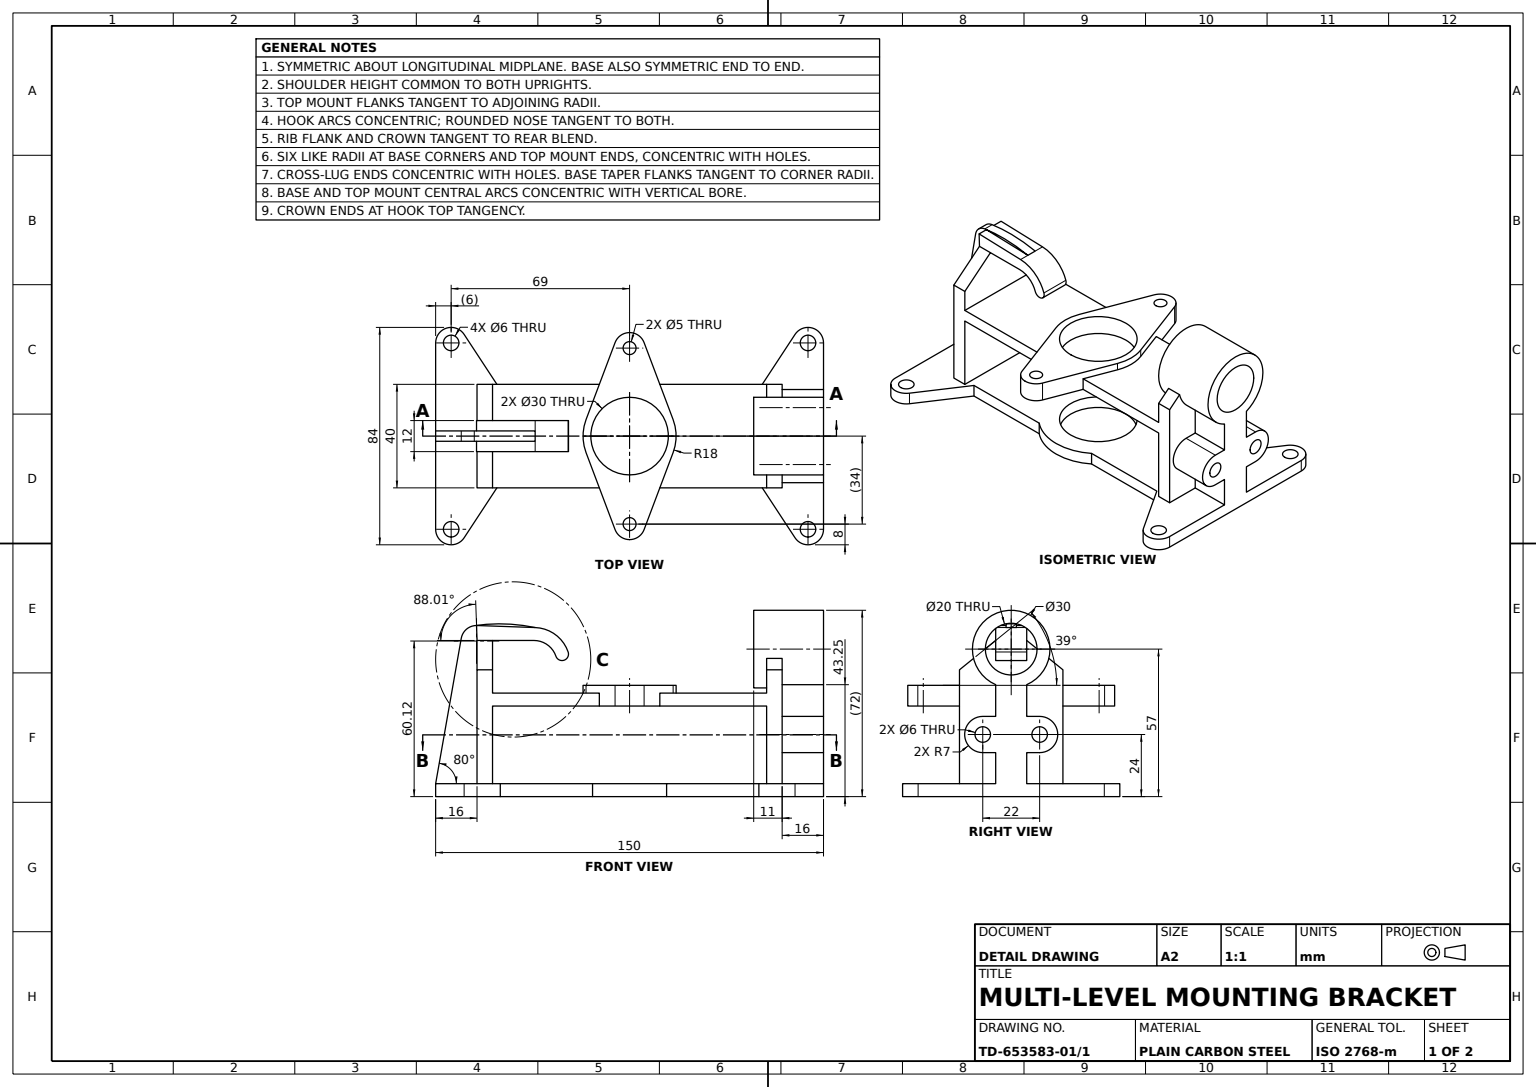
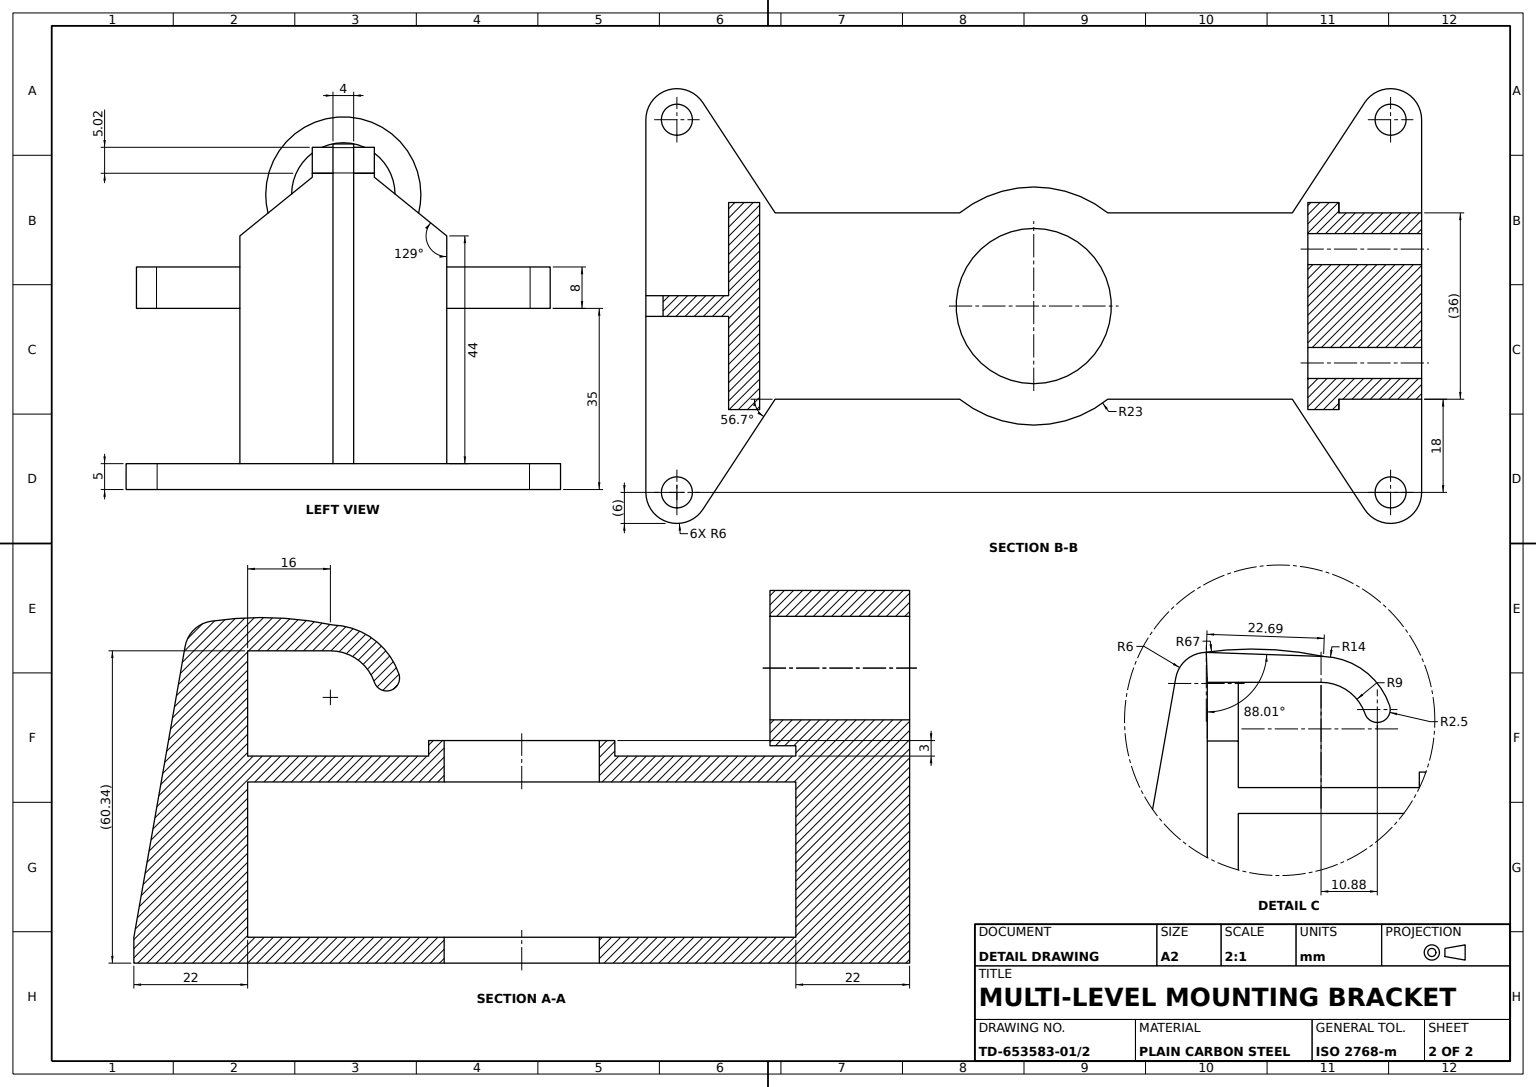
from build123d import *
from build123d.topology import SkipClean

# Parameters (mm, degrees)
BASE_PLATE_SKETCH_R           = 15
BASE_PLATE_SKETCH_R_2         = 3
BASE_PLATE_DEPTH              = 5
CENTER_PEDESTAL_SKETCH_W      = 6
CENTER_PEDESTAL_SKETCH_H      = 40
CENTER_PEDESTAL_DEPTH         = 44
MID_FLANGE_PLATE_DEPTH        = 6
MID_FLANGE_BOSS_11MM_DEPTH    = 11
FLANGE_START                  = 16
FLANGE_WEB_SKETCH_R           = 10
FLANGE_WEB_DEPTH              = 16
CENTER_BORE_SKETCH_R          = 10
CENTER_BORE_CUT_DEPTH         = 50
UPPER_BRACKET_SKETCH_W        = 12
UPPER_BRACKET_SKETCH_H        = 11.336976465
UPPER_BRACKET_SKETCH_W_2      = 14
UPPER_BRACKET_SKETCH_H_2      = 44
UPPER_BRACKET_SKETCH_H_3      = 5
UPPER_BRACKET_PLATE_DEPTH     = 6
SKETCH6_3_W                   = 12
SKETCH6_3_H                   = 2
UPPER_BRACKET_WALL_22MM_DEPTH = 22
SUPPORT_RIB_DEPTH             = 2
SIDE_BRACKET_BLOCK_12MM_DEPTH = 6
SIDE_BRACKET_LIP_4MM_DEPTH    = 2
TOP_MOUNT_SKETCH_W            = 118
TOP_MOUNT_SKETCH_H            = 40
TOP_MOUNT_SKETCH_R            = 15
TOP_MOUNT_PLATE_5MM_DEPTH     = 5
SKETCH9_3_R                   = 6
SKETCH9_3_R_2                 = 2.5
SKETCH9_3_R_3                 = 18
SKETCH9_3_R_4                 = 15
TOP_MOUNT_TABS_8MM_DEPTH      = 8
TUBE_BOSS_SKETCH_R            = 3
TUBE_BOSS_DEPTH               = 16
TUBE_BORE_SKETCH_R            = 3
TUBE_BORE_CUT_DEPTH           = 50


with BuildPart() as part:
    # Base Plate Sketch → Base Plate (new body)
    with BuildSketch(Plane(origin=(0, 0, 0), x_dir=(1, 0, 0), z_dir=(0, 1, 0))):
        with BuildLine():
            Line((14.317821063, 18), (50, 18))
            Line((50, 18), (63.984888076, 39.293729253))
            ThreePointArc((63.984888076, 39.293729253), (70.718913677, 41.748507265), (75, 36))
            Line((75, 36), (75, -36))
            ThreePointArc((75, -36), (70.718913677, -41.748507265), (63.984888076, -39.293729253))
            Line((63.984888076, -39.293729253), (50, -18))
            Line((50, -18), (14.317821063, -18))
            ThreePointArc((14.317821063, -18), (0, -23), (-14.317821063, -18))
            Line((-14.317821063, -18), (-50, -18))
            Line((-50, -18), (-63.984888076, -39.293729253))
            ThreePointArc((-63.984888076, -39.293729253), (-70.718913677, -41.748507265), (-75, -36))
            Line((-75, -36), (-75, 36))
            ThreePointArc((-75, 36), (-70.718913677, 41.748507265), (-63.984888076, 39.293729253))
            Line((-63.984888076, 39.293729253), (-50, 18))
            Line((-50, 18), (-14.317821063, 18))
            ThreePointArc((-14.317821063, 18), (0, 23), (14.317821063, 18))
        make_face()
        with Locations(Location((0, 0, 0), (0, 0, 270))):
            Circle(BASE_PLATE_SKETCH_R, mode=Mode.SUBTRACT)
        with Locations(Location((-69, 36, 0), (0, 0, 270))):
            Circle(BASE_PLATE_SKETCH_R_2, mode=Mode.SUBTRACT)
        with Locations(Location((-69, -36, 0), (0, 0, 270))):
            Circle(BASE_PLATE_SKETCH_R_2, mode=Mode.SUBTRACT)
        with Locations(Location((69, 36, 0), (0, 0, 270))):
            Circle(BASE_PLATE_SKETCH_R_2, mode=Mode.SUBTRACT)
        with Locations(Location((69, -36, 0), (0, 0, 270))):
            Circle(BASE_PLATE_SKETCH_R_2, mode=Mode.SUBTRACT)
    extrude(amount=BASE_PLATE_DEPTH)

    # Center Pedestal Sketch → Center Pedestal (add)
    with BuildSketch(Plane(origin=(0, 5, 0), x_dir=(1, 0, 0), z_dir=(0, 1, 0))):
        with Locations((-56, 0)):
            Rectangle(CENTER_PEDESTAL_SKETCH_W, CENTER_PEDESTAL_SKETCH_H)
        with Locations((56, 0)):
            Rectangle(CENTER_PEDESTAL_SKETCH_W, CENTER_PEDESTAL_SKETCH_H)
    extrude(amount=CENTER_PEDESTAL_DEPTH)

    # Mid Flange Sketch → Mid Flange Plate (add)
    with BuildSketch(Plane.ZY.offset(59)):
        with BuildLine():
            ThreePointArc((6.545818153, 70.496379689), (-9.439805866, 68.657189422), (-14.562403531, 53.403278799))
            ThreePointArc((-14.562403531, 53.403278799), (-13.802217517, 51.126432803), (-12.68857754, 49))
            Line((-12.68857754, 49), (-6, 49))
            ThreePointArc((-6, 49), (-4.472135955, 65.94427191), (10, 57))
            ThreePointArc((10, 57), (8.94427191, 52.527864045), (6, 49))
            Line((6, 49), (12.68857754, 49))
            ThreePointArc((12.68857754, 49), (13.802217517, 51.126432803), (14.562403531, 53.403278799))
            ThreePointArc((14.562403531, 53.403278799), (14.890199008, 55.188378208), (15, 57))
            ThreePointArc((15, 57), (12.711948558, 64.962811303), (6.545818153, 70.496379689))
        make_face()
        with BuildLine():
            Line((-6, 49), (-12.68857754, 49))
            ThreePointArc((-12.68857754, 49), (0, 42), (12.68857754, 49))
            Line((12.68857754, 49), (6, 49))
            ThreePointArc((6, 49), (0, 47), (-6, 49))
        make_face()
        with BuildLine():
            Line((-14.562403531, 53.403278799), (-20, 49))
            Line((-20, 49), (-12.68857754, 49))
            ThreePointArc((-12.68857754, 49), (-13.802217517, 51.126432803), (-14.562403531, 53.403278799))
        make_face()
        with BuildLine():
            ThreePointArc((6.545818153, 70.496379689), (-9.439805866, 68.657189422), (-14.562403531, 53.403278799))
            ThreePointArc((-14.562403531, 53.403278799), (-13.802217517, 51.126432803), (-12.68857754, 49))
            Line((-12.68857754, 49), (-6, 49))
            ThreePointArc((-6, 49), (-4.472135955, 65.94427191), (10, 57))
            ThreePointArc((10, 57), (8.94427191, 52.527864045), (6, 49))
            Line((6, 49), (12.68857754, 49))
            ThreePointArc((12.68857754, 49), (13.802217517, 51.126432803), (14.562403531, 53.403278799))
            ThreePointArc((14.562403531, 53.403278799), (14.890199008, 55.188378208), (15, 57))
            ThreePointArc((15, 57), (12.711948558, 64.962811303), (6.545818153, 70.496379689))
        make_face()
        with BuildLine():
            Line((-6, 49), (-12.68857754, 49))
            ThreePointArc((-12.68857754, 49), (0, 42), (12.68857754, 49))
            Line((12.68857754, 49), (6, 49))
            ThreePointArc((6, 49), (0, 47), (-6, 49))
        make_face()
        with BuildLine():
            ThreePointArc((14.562403531, 53.403278799), (13.802217517, 51.126432803), (12.68857754, 49))
            Line((12.68857754, 49), (20, 49))
            Line((20, 49), (14.562403531, 53.403278799))
        make_face()
    extrude(amount=-MID_FLANGE_PLATE_DEPTH)

    # Sketch3_3 → Mid Flange Boss 11mm (add)
    with BuildSketch(Plane.ZY.offset(59)):
        with BuildLine():
            ThreePointArc((6.545818153, 70.496379689), (-9.439805866, 68.657189422), (-14.562403531, 53.403278799))
            ThreePointArc((-14.562403531, 53.403278799), (-13.802217517, 51.126432803), (-12.68857754, 49))
            Line((-12.68857754, 49), (-6, 49))
            ThreePointArc((-6, 49), (-4.472135955, 65.94427191), (10, 57))
            ThreePointArc((10, 57), (8.94427191, 52.527864045), (6, 49))
            Line((6, 49), (12.68857754, 49))
            ThreePointArc((12.68857754, 49), (13.802217517, 51.126432803), (14.562403531, 53.403278799))
            ThreePointArc((14.562403531, 53.403278799), (14.890199008, 55.188378208), (15, 57))
            ThreePointArc((15, 57), (12.711948558, 64.962811303), (6.545818153, 70.496379689))
        make_face()
        with BuildLine():
            Line((-6, 49), (-12.68857754, 49))
            ThreePointArc((-12.68857754, 49), (0, 42), (12.68857754, 49))
            Line((12.68857754, 49), (6, 49))
            ThreePointArc((6, 49), (0, 47), (-6, 49))
        make_face()
        with BuildLine():
            ThreePointArc((6.545818153, 70.496379689), (-9.439805866, 68.657189422), (-14.562403531, 53.403278799))
            ThreePointArc((-14.562403531, 53.403278799), (-13.802217517, 51.126432803), (-12.68857754, 49))
            Line((-12.68857754, 49), (-6, 49))
            ThreePointArc((-6, 49), (-4.472135955, 65.94427191), (10, 57))
            ThreePointArc((10, 57), (8.94427191, 52.527864045), (6, 49))
            Line((6, 49), (12.68857754, 49))
            ThreePointArc((12.68857754, 49), (13.802217517, 51.126432803), (14.562403531, 53.403278799))
            ThreePointArc((14.562403531, 53.403278799), (14.890199008, 55.188378208), (15, 57))
            ThreePointArc((15, 57), (12.711948558, 64.962811303), (6.545818153, 70.496379689))
        make_face()
        with BuildLine():
            Line((-6, 49), (-12.68857754, 49))
            ThreePointArc((-12.68857754, 49), (0, 42), (12.68857754, 49))
            Line((12.68857754, 49), (6, 49))
            ThreePointArc((6, 49), (0, 47), (-6, 49))
        make_face()
    extrude(amount=-MID_FLANGE_BOSS_11MM_DEPTH)

    # Flange Web Sketch → Flange Web (add)
    with SkipClean():  # the faces are left unmerged after this step: merging them gives an invalid solid
        with BuildSketch(Plane.ZY.offset(59).offset(FLANGE_START)):
            with BuildLine():
                Line((-6, 0), (6, 0))
                Line((6, 0), (6, 43.252272915))
                ThreePointArc((6, 43.252272915), (0, 72), (-6, 43.252272915))
                Line((-6, 43.252272915), (-6, 0))
            make_face()
            with Locations((0, 57)):
                Circle(FLANGE_WEB_SKETCH_R, mode=Mode.SUBTRACT)
        extrude(amount=-FLANGE_WEB_DEPTH)

    # Center Bore Sketch → Center Bore Cut (cut)
    with SkipClean():  # the faces are left unmerged after this step: merging them gives an invalid solid
        with BuildSketch(Plane.ZY.offset(75)):
            with Locations((0, 57)):
                Circle(CENTER_BORE_SKETCH_R)
        extrude(amount=-CENTER_BORE_CUT_DEPTH, mode=Mode.SUBTRACT)

    # Upper Bracket Sketch → Upper Bracket Plate (add)
    with SkipClean():  # the faces are left unmerged after this step: merging them gives an invalid solid
        with BuildSketch(Plane(origin=(59, 0, 0), x_dir=(0, 0, -1), z_dir=(1, 0, 0))):
            with Locations((0, 54.668488233)):
                Rectangle(UPPER_BRACKET_SKETCH_W, UPPER_BRACKET_SKETCH_H)
            Polygon((-20, 49), (-6, 49), (-6, 60.336976465), align=None)
            Polygon((6, 60.336976465), (6, 49), (20, 49), align=None)
            with Locations((-13, 27)):
                Rectangle(UPPER_BRACKET_SKETCH_W_2, UPPER_BRACKET_SKETCH_H_2)
            with Locations((0, 27)):
                Rectangle(UPPER_BRACKET_SKETCH_W, UPPER_BRACKET_SKETCH_H_2)
            with Locations((13, 27)):
                Rectangle(UPPER_BRACKET_SKETCH_W_2, UPPER_BRACKET_SKETCH_H_2)
            with Locations((0, 2.5)):
                Rectangle(UPPER_BRACKET_SKETCH_W, UPPER_BRACKET_SKETCH_H_3)
        extrude(amount=-UPPER_BRACKET_PLATE_DEPTH)

    # Sketch6_3 → Upper Bracket Wall 22mm (add)
    with SkipClean():  # the faces are left unmerged after this step: merging them gives an invalid solid
        with BuildSketch(Plane(origin=(59, 0, 0), x_dir=(0, 0, -1), z_dir=(1, 0, 0))):
            with Locations((0, 61.336976465)):
                Rectangle(SKETCH6_3_W, SKETCH6_3_H)
        extrude(amount=-UPPER_BRACKET_WALL_22MM_DEPTH)

    # Support Rib Sketch → Support Rib (add, symmetric)
    with SkipClean():  # the faces are left unmerged after this step: merging them gives an invalid solid
        with BuildSketch(Plane.XY):
            with BuildLine():
                Line((75, 5), (65.097528939, 61.159704097))
                ThreePointArc((65.097528939, 61.159704097), (63.045408079, 64.714081689), (59.188682421, 66.117815031))
                ThreePointArc((59.188682421, 66.117815031), (47.934434691, 65.165842314), (37, 62.336976465))
                Line((37, 62.336976465), (59, 62.336976465))
                Line((59, 62.336976465), (59, 5))
                Line((59, 5), (75, 5))
            make_face()
        extrude(amount=SUPPORT_RIB_DEPTH, both=True)

    # Side Bracket Sketch → Side Bracket Block 12mm (add, symmetric)
    with SkipClean():  # the faces are left unmerged after this step: merging them gives an invalid solid
        with BuildSketch(Plane.XY):
            with BuildLine():
                Line((36.512972901, 65.328502636), (59.188682421, 66.117815031))
                Line((59.188682421, 66.117815031), (59.014780713, 61.103282774))
                Line((59.014780713, 61.103282774), (37, 60.336976465))
                ThreePointArc((37, 60.336976465), (31.771489867, 58.662458141), (28.488587739, 54.262016862))
                ThreePointArc((28.488587739, 54.262016862), (25.311795334, 52.7102469), (23.760025372, 55.887039305))
                ThreePointArc((23.760025372, 55.887039305), (28.669756813, 62.588956221), (36.512972901, 65.328502636))
            make_face()
        extrude(amount=SIDE_BRACKET_BLOCK_12MM_DEPTH, both=True)

    # Sketch8_6 → Side Bracket Lip 4mm (add, symmetric)
    with SkipClean():  # the faces are left unmerged after this step: merging them gives an invalid solid
        with BuildSketch(Plane.XY):
            with BuildLine():
                ThreePointArc((60.061181917, 66.054038125), (63.370223983, 64.420687346), (65.097528939, 61.159704097))
                Line((65.097528939, 61.159704097), (75, 5))
                Line((75, 5), (59, 5))
                Line((59, 5), (59.188682421, 66.117815031))
                Line((59.188682421, 66.117815031), (36.512972901, 65.328502636))
                ThreePointArc((36.512972901, 65.328502636), (48.254936842, 66.734434783), (60.061181917, 66.054038125))
            make_face()
        extrude(amount=SIDE_BRACKET_LIP_4MM_DEPTH, both=True)

    # Top Mount Sketch → Top Mount Plate 5mm (add)
    with SkipClean():  # the faces are left unmerged after this step: merging them gives an invalid solid
        with BuildSketch(Plane(origin=(0, 35, 0), x_dir=(1, 0, 0), z_dir=(0, 1, 0))):
            Rectangle(TOP_MOUNT_SKETCH_W, TOP_MOUNT_SKETCH_H)
            with Locations(Location((0, 0, 0), (0, 0, 270))):
                Circle(TOP_MOUNT_SKETCH_R, mode=Mode.SUBTRACT)
        extrude(amount=TOP_MOUNT_PLATE_5MM_DEPTH)

    # Sketch9_3 → Top Mount Tabs 8mm (add)
    # profile 1 of 7: a face of its own
    with SkipClean():  # the faces are left unmerged after this step: merging them gives an invalid solid
        with BuildSketch(Plane(origin=(0, 35, 0), x_dir=(1, 0, 0), z_dir=(0, 1, 0))):
            with Locations((0, 34)):
                Circle(SKETCH9_3_R)
            with Locations(Location((0, 34, 0), (0, 0, 270))):
                Circle(SKETCH9_3_R_2, mode=Mode.SUBTRACT)
        # profile 2 of 7: a face of its own
        with BuildSketch(Plane(origin=(0, 35, 0), x_dir=(1, 0, 0), z_dir=(0, 1, 0))):
            with BuildLine():
                Line((-5.613873078, 36.117647059), (-11.69371981, 20))
                Line((-11.69371981, 20), (11.69371981, 20))
                Line((11.69371981, 20), (5.613873078, 36.117647059))
                ThreePointArc((5.613873078, 36.117647059), (5.902678988, 35.076280989), (6, 34))
                ThreePointArc((6, 34), (-1.076280989, 28.097321012), (-5.613873078, 36.117647059))
            make_face()
        # profile 3 of 7: a face of its own
        with BuildSketch(Plane(origin=(0, 35, 0), x_dir=(1, 0, 0), z_dir=(0, 1, 0))):
            Circle(SKETCH9_3_R_3)
            with Locations(Location((0, 0, 0), (0, 0, 270))):
                Circle(SKETCH9_3_R_4, mode=Mode.SUBTRACT)
        # profile 4 of 7: a face of its own
        with BuildSketch(Plane(origin=(0, 35, 0), x_dir=(1, 0, 0), z_dir=(0, 1, 0))):
            with BuildLine():
                Line((11.69371981, 20), (-11.69371981, 20))
                Line((-11.69371981, 20), (-16.841619234, 6.352941176))
                ThreePointArc((-16.841619234, 6.352941176), (0, 18), (16.841619234, 6.352941176))
                Line((16.841619234, 6.352941176), (11.69371981, 20))
            make_face()
        # profile 5 of 7: a face of its own
        with BuildSketch(Plane(origin=(0, 35, 0), x_dir=(1, 0, 0), z_dir=(0, 1, 0))):
            with BuildLine():
                Line((-16.841619234, -6.352941176), (-11.69371981, -20))
                Line((-11.69371981, -20), (11.69371981, -20))
                Line((11.69371981, -20), (16.841619234, -6.352941176))
                ThreePointArc((16.841619234, -6.352941176), (0, -18), (-16.841619234, -6.352941176))
            make_face()
        # profile 6 of 7: a face of its own
        with BuildSketch(Plane(origin=(0, 35, 0), x_dir=(1, 0, 0), z_dir=(0, 1, 0))):
            with BuildLine():
                Line((11.69371981, -20), (-11.69371981, -20))
                Line((-11.69371981, -20), (-5.613873078, -36.117647059))
                ThreePointArc((-5.613873078, -36.117647059), (-1.076280989, -28.097321012), (6, -34))
                ThreePointArc((6, -34), (5.902678988, -35.076280989), (5.613873078, -36.117647059))
                Line((5.613873078, -36.117647059), (11.69371981, -20))
            make_face()
        # profile 7 of 7: a face of its own
        with BuildSketch(Plane(origin=(0, 35, 0), x_dir=(1, 0, 0), z_dir=(0, 1, 0))):
            with Locations((0, -34)):
                Circle(SKETCH9_3_R)
            with Locations(Location((0, -34, 0), (0, 0, 270))):
                Circle(SKETCH9_3_R_2, mode=Mode.SUBTRACT)
        extrude(amount=TOP_MOUNT_TABS_8MM_DEPTH)

    # Tube Boss Sketch → Tube Boss (add)
    # profile 1 of 9: a face of its own
    with SkipClean():  # the faces are left unmerged after this step: merging them gives an invalid solid
        with BuildSketch(Plane.ZY.offset(75)):
            with BuildLine():
                ThreePointArc((-6, 28.898979486), (-8.288252998, 30.453404388), (-11, 31))
                ThreePointArc((-11, 31), (-18, 24), (-11, 17))
                ThreePointArc((-11, 17), (-8.288252998, 17.546595612), (-6, 19.101020514))
                Line((-6, 19.101020514), (-6, 28.898979486))
            make_face()
            with Locations((-11, 24)):
                Circle(TUBE_BOSS_SKETCH_R, mode=Mode.SUBTRACT)
        # profile 2 of 9: a face of its own
        with BuildSketch(Plane.ZY.offset(75)):
            with BuildLine():
                Line((6, 31), (-6, 31))
                Line((-6, 31), (-6, 28.898979486))
                ThreePointArc((-6, 28.898979486), (-4.519259302, 26.645751311), (-4, 24))
                ThreePointArc((-4, 24), (-4.519259302, 21.354248689), (-6, 19.101020514))
                Line((-6, 19.101020514), (-6, 17))
                Line((-6, 17), (6, 17))
                Line((6, 17), (6, 19.101020514))
                ThreePointArc((6, 19.101020514), (4, 24), (6, 28.898979486))
                Line((6, 28.898979486), (6, 31))
            make_face()
        # profile 3 of 9: a face of its own
        with BuildSketch(Plane.ZY.offset(75)):
            with BuildLine():
                Line((-6, 31), (-11, 31))
                ThreePointArc((-11, 31), (-8.288252998, 30.453404388), (-6, 28.898979486))
                Line((-6, 28.898979486), (-6, 31))
            make_face()
        # profile 4 of 9: a face of its own
        with BuildSketch(Plane.ZY.offset(75)):
            with BuildLine():
                ThreePointArc((-4, 24), (-4.519259302, 26.645751311), (-6, 28.898979486))
                Line((-6, 28.898979486), (-6, 19.101020514))
                ThreePointArc((-6, 19.101020514), (-4.519259302, 21.354248689), (-4, 24))
            make_face()
        # profile 5 of 9: a face of its own
        with BuildSketch(Plane.ZY.offset(75)):
            with BuildLine():
                ThreePointArc((-6, 19.101020514), (-8.288252998, 17.546595612), (-11, 17))
                Line((-11, 17), (-6, 17))
                Line((-6, 17), (-6, 19.101020514))
            make_face()
        # profile 6 of 9: a face of its own
        with BuildSketch(Plane.ZY.offset(75)):
            with BuildLine():
                Line((6, 19.101020514), (6, 28.898979486))
                ThreePointArc((6, 28.898979486), (4, 24), (6, 19.101020514))
            make_face()
        # profile 7 of 9: a face of its own
        with BuildSketch(Plane.ZY.offset(75)):
            with BuildLine():
                ThreePointArc((18, 24), (15.949747468, 28.949747468), (11, 31))
                ThreePointArc((11, 31), (8.288252998, 30.453404388), (6, 28.898979486))
                Line((6, 28.898979486), (6, 19.101020514))
                ThreePointArc((6, 19.101020514), (8.288252998, 17.546595612), (11, 17))
                ThreePointArc((11, 17), (15.949747468, 19.050252532), (18, 24))
            make_face()
            with Locations((11, 24)):
                Circle(TUBE_BOSS_SKETCH_R, mode=Mode.SUBTRACT)
        # profile 8 of 9: a face of its own
        with BuildSketch(Plane.ZY.offset(75)):
            with BuildLine():
                Line((6, 19.101020514), (6, 17))
                Line((6, 17), (11, 17))
                ThreePointArc((11, 17), (8.288252998, 17.546595612), (6, 19.101020514))
            make_face()
        # profile 9 of 9: a face of its own
        with BuildSketch(Plane.ZY.offset(75)):
            with BuildLine():
                Line((11, 31), (6, 31))
                Line((6, 31), (6, 28.898979486))
                ThreePointArc((6, 28.898979486), (8.288252998, 30.453404388), (11, 31))
            make_face()
        extrude(amount=-TUBE_BOSS_DEPTH)

    # Tube Bore Sketch → Tube Bore Cut (cut)
    with SkipClean():  # the faces are left unmerged after this step: merging them gives an invalid solid
        with BuildSketch(Plane.ZY.offset(75)):
            with Locations((-11, 24)):
                Circle(TUBE_BORE_SKETCH_R)
            with Locations((11, 24)):
                Circle(TUBE_BORE_SKETCH_R)
        extrude(amount=-TUBE_BORE_CUT_DEPTH, mode=Mode.SUBTRACT)


solid = part.part
